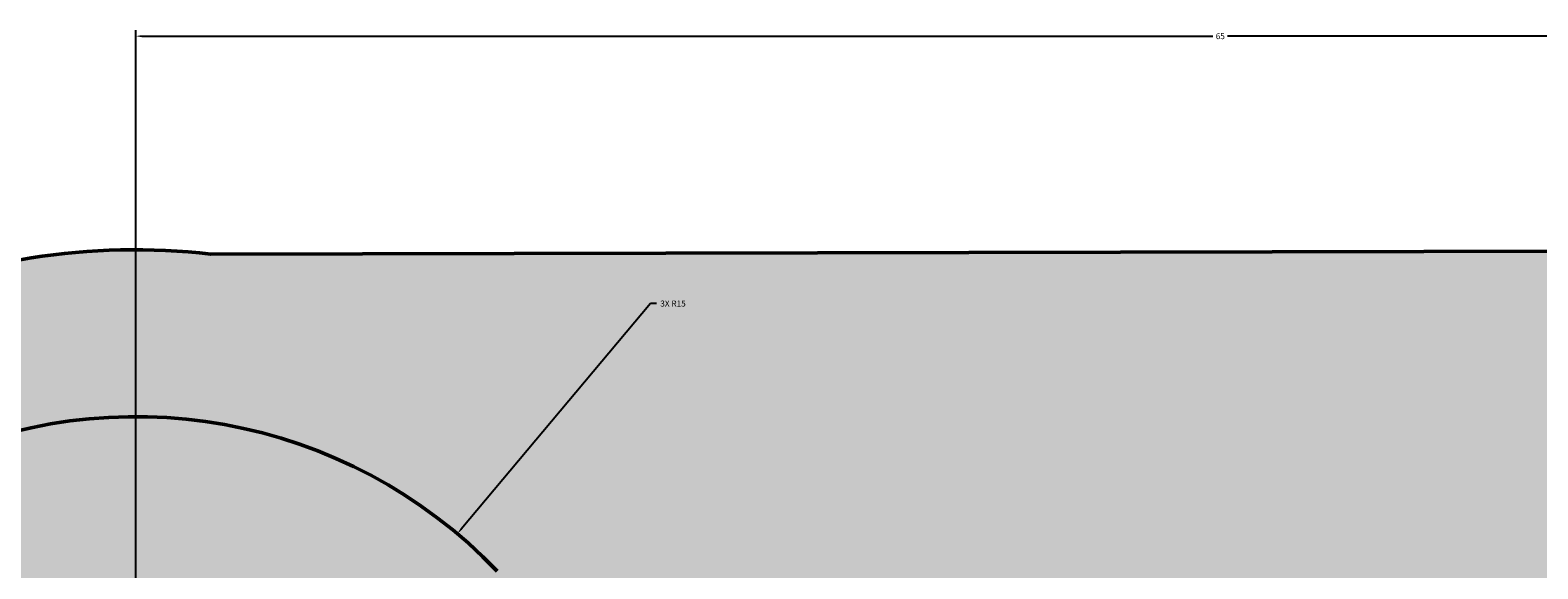
# Model space of a CAD drawing. Units: inches. Extents: x -31 to 87, y -18 to 100.
# Tile 6 of 7: x -8 to 37, y 84 to 100. Entities that reach past the tile are written whole.
import ezdxf

# ---------------------------------------------------------------- set-up
doc = ezdxf.new("R2010")
doc.units = ezdxf.units.IN
doc.header["$MEASUREMENT"] = 0
for name, color, linetype, lineweight in [('M-DIMS', 2, 'Continuous', 18), ('M-HATC', 7, 'Continuous', 18), ('M-OUTL', 4, 'Continuous', 50)]:
    doc.layers.add(name, color=color, linetype=linetype, lineweight=lineweight)
doc.styles.get("Standard").update_dxf_attribs({"font": 'arial.ttf'})
doc.dimstyles.get("Standard").update_dxf_attribs({"dimtxt": 0.18, "dimasz": 0.18, "dimexe": 0.18, "dimexo": 0.0625, "dimgap": 0.09, "dimtad": 0, "dimtih": 1, "dimtoh": 1, "dimdec": 4, "dimzin": 0, "dimdsep": 46, "dimtxsty": 'Standard', "dimcen": 0.09, "dimadec": 0, "dimazin": 0, "dimtfac": 1, "dimtdec": 4, "dimtofl": 0, "dimtmove": 0, "dimatfit": 3, "dimfxl": 1, "dimtolj": 1, "dimtzin": 0, "dimarcsym": 0})

# ---------------------------------------------------------------- blocks, each defined once
blk = doc.blocks.new('*D2')
at = {"layer": 'Defpoints', "color": 0, "transparency": 16777216}
for p in [(60.278, 93.49), (86.68, 93.49), (28.858, -11.451)]:
    blk.add_point(p, dxfattribs=at)
at = {"layer": 'M-DIMS', "color": 0, "lineweight": -2, "transparency": 16777216}
for p, q in [((60.341, 93.49), (86.86, 93.49)), ((86.68, 93.31), (86.68, 41.201)), ((86.68, -11.271), (86.68, 40.838)), ((28.92, -11.451), (86.86, -11.451))]:
    blk.add_line(p, q, dxfattribs=at)
at = {"layer": 'M-DIMS', "color": 0, "transparency": 16777216}
for points in [[(86.65, 93.31), (86.71, 93.31), (86.68, 93.49)], [(86.65, -11.271), (86.71, -11.271), (86.68, -11.451)]]:
    blk.add_solid(points, dxfattribs=at)
at = {"layer": 'M-DIMS', "color": 0, "transparency": 16777216, "insert": (86.68, 41.019), "char_height": 0.18, "attachment_point": 5}
blk.add_mtext('\\A1;104.94', dxfattribs=at)
blk = doc.blocks.new('*D3')
at = {"layer": 'Defpoints', "color": 0, "transparency": 16777216}
for p in [(60.319, 99.89), (-4.681, 73.49), (60.319, 73.49)]:
    blk.add_point(p, dxfattribs=at)
at = {"layer": 'M-DIMS', "color": 0, "lineweight": -2, "transparency": 16777216}
for p, q in [((-4.681, 73.552), (-4.681, 100.07)), ((-4.501, 99.89), (27.599, 99.89)), ((60.139, 99.89), (28.039, 99.89)), ((60.319, 73.552), (60.319, 100.07))]:
    blk.add_line(p, q, dxfattribs=at)
at = {"layer": 'M-DIMS', "color": 0, "transparency": 16777216}
for points in [[(-4.501, 99.92), (-4.501, 99.86), (-4.681, 99.89)], [(60.139, 99.92), (60.139, 99.86), (60.319, 99.89)]]:
    blk.add_solid(points, dxfattribs=at)
at = {"layer": 'M-DIMS', "color": 0, "transparency": 16777216, "insert": (27.819, 99.89), "char_height": 0.18, "attachment_point": 5}
blk.add_mtext('\\A1;65', dxfattribs=at)
blk = doc.blocks.new('*D8')
at = {"layer": 'Defpoints', "color": 0, "transparency": 16777216}
for p in [(4.958, 84.983), (-4.681, 73.49)]:
    blk.add_point(p, dxfattribs=at)
at = {"layer": 'M-DIMS', "color": 0, "lineweight": -2, "transparency": 16777216}
for p, q in [((10.741, 91.879), (5.073, 85.121)), ((10.921, 91.879), (10.741, 91.879)), ((-4.771, 73.49), (-4.591, 73.49)), ((-4.681, 73.4), (-4.681, 73.58))]:
    blk.add_line(p, q, dxfattribs=at)
at = {"layer": 'M-DIMS', "color": 0, "transparency": 16777216}
blk.add_solid([(5.05, 85.14), (5.096, 85.102), (4.958, 84.983)], dxfattribs=at)
at = {"layer": 'M-DIMS', "color": 0, "transparency": 16777216, "insert": (11.42, 91.879), "char_height": 0.18, "attachment_point": 5}
blk.add_mtext('\\A1;3X R15', dxfattribs=at)

msp = doc.modelspace()

# ---------------------------------------------------------------- hatches: boundary and pattern name
at = {"layer": 'M-HATC'}
h = msp.add_hatch(color=256, dxfattribs=at)
h.set_gradient(color1=(205, 32, 39), color2=(247, 242, 129))
h.paths.add_polyline_path([(-2.425, 93.362, 0.593504), (-22.614, 64.635), (8.64, 1.342, 0.746388), (46.874, 4.293), (79.436, 67.614, 0.505151), (60.278, 93.49)])
h.paths.add_polyline_path([(49.486, 83.865, -1.392259), (62.663, 58.674, 0.510547), (40.663, 15.341, -1.641082), (14.002, 15.393, 0.505248), (-7.332, 58.726, -1.377138), (6.152, 83.865, 0.426931)], flags=16)
h.paths.add_polyline_path([(5.319, 73.49, -1), (-14.681, 73.49, -1)], flags=0)
h.paths.add_polyline_path([(70.319, 73.49, -1), (50.319, 73.49, -1)], flags=0)
h.paths.add_polyline_path([(37.319, 8.49, -1), (17.319, 8.49, -1)], flags=0)
h.paths.add_polyline_path([(6.152, 83.865, 1.377138), (-7.332, 58.726, -0.505248), (14.002, 15.393, 1.641082), (40.663, 15.341, -0.510547), (62.663, 58.674, 1.392259), (49.486, 83.865, -0.426931)], flags=0)

# ---------------------------------------------------------------- linework, layer by layer
at = {"layer": 'M-OUTL'}
msp.add_line((-2.425, 93.362), (60.278, 93.49), dxfattribs=at)
for radius, start, end in [(20, 83.5229, 206.2801), (15, 43.7617, 259.8216)]:
    msp.add_arc((-4.681, 73.49), radius, start, end, dxfattribs=at)

# ---------------------------------------------------------------- dimensions: what is measured, and where the dimension line sits
at = {"layer": 'M-DIMS'}
dim = msp.add_linear_dim(base=(60.319, 99.89), p1=(-4.681, 73.49), p2=(60.319, 73.49), dimstyle='Standard', override={"dimdec": 0, "dimlfac": 1, "dimrnd": 0, "dimzin": 0, "dimdsep": 46, "dimlunit": 2}, dxfattribs=at)
dim.commit()
dim.dimension.update_dxf_attribs({"geometry": '*D3', "text_midpoint": (27.819, 99.89)})
dim = msp.add_linear_dim(base=(86.68, 93.49), p1=(28.858, -11.451), p2=(60.278, 93.49), angle=90, dimstyle='Standard', override={"dimdec": 2, "dimlfac": 1, "dimrnd": 0, "dimzin": 0, "dimdsep": 46, "dimlunit": 2}, dxfattribs=at)
dim.commit()
dim.dimension.update_dxf_attribs({"geometry": '*D2', "text_midpoint": (86.68, 41.019)})
dim = msp.add_radius_dim(center=(-4.681, 73.49), mpoint=(4.958, 84.983), text='3X <>', dimstyle='Standard', override={"dimdec": 0, "dimlfac": 1, "dimrnd": 0, "dimzin": 0, "dimdsep": 46, "dimlunit": 2}, dxfattribs=at)
dim.commit()
dim.dimension.update_dxf_attribs({"geometry": '*D8', "text_midpoint": (11.42, 91.879), "dimtype": 164})

doc.saveas('drawing.dxf')
